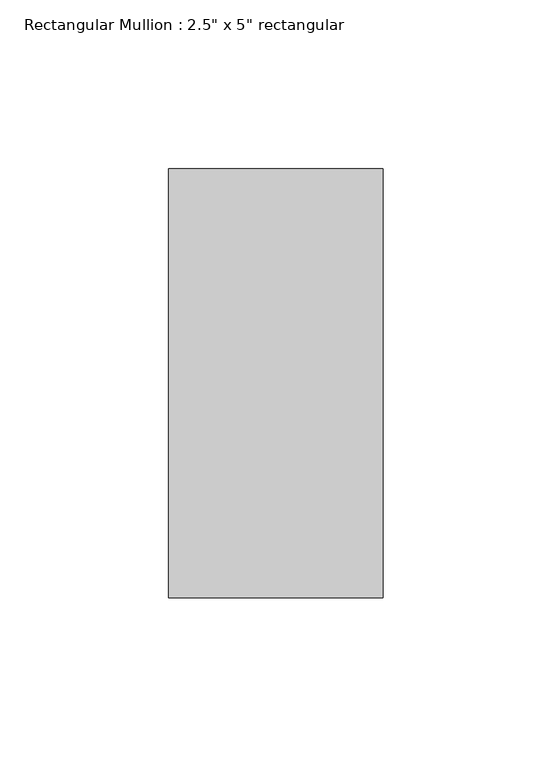
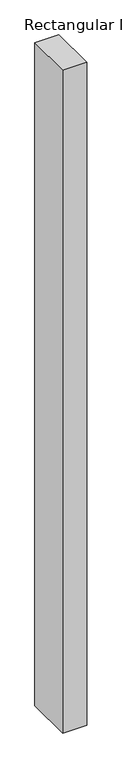
"""IFC4 building model written with IfcOpenShell, lengths in millimetres: member geometry."""

from ifc_helpers import new_model, si_unit, frame, origin, place, context, project, spatial, polyline, outline, extrude, source, transform, mapped, element, save


def member_51608f29(model_context):
    return source(origin(), model_context, "Body", "SweptSolid", [
        extrude(outline(polyline([(0.0, 63.5), (0.0, -63.5), (-63.5, -63.5), (-63.5, 63.5), (0.0, 63.5)])), frame((0.0, 0.0, -1852.7814546), z_axis=(0.0, 0.0, 1.0), x_axis=(1.0, 0.0, 0.0)), (0.0, 0.0, 1.0), 1852.7814546),
    ])


if __name__ == "__main__":
    model = new_model("IFC4")
    model_context = context("Model", 3, world=origin())
    ifc_project = project(units=[si_unit("LENGTHUNIT", "METRE", prefix="MILLI")], contexts=[model_context])
    site = spatial("IfcSite", under=ifc_project)
    building = spatial("IfcBuilding", under=site)
    placement = place(None, origin())
    member_shape = member_51608f29(model_context)
    element("IfcMember", 1, ObjectType="Rectangular Mullion : 2.5\" x 5\" rectangular", at=placement, inside=building, context=model_context, shape_type="MappedRepresentation", body=[
        mapped(member_shape, transform((0.0, 0.0, 0.0), x_axis=(1.0, 0.0, 0.0), y_axis=(0.0, 1.0, 0.0), z_axis=(0.0, 0.0, 1.0))),
    ])
    save(model, "model.ifc")

# Revit data of these elements
# Type "Rectangular Mullion : 2.5\" x 5\" rectangular"
#   built-in parameter 1007304 = 0.416667 (stored number, unit not read)
#   built-in parameter 1007301 = 0.104167 (stored number, unit not read)
#   built-in parameter 1007300 = 0.104167 (stored number, unit not read)
# Element 1 (IfcMember, "Rectangular Mullion : 2.5\" x 5\" rectangular")
#   Materials on its faces: "Aluminum"
# Materials
#   "Aluminum": class "Metal", colour RGB 247 247 247, transparency 0, Description = "Aluminum 6061", Cost = 0
